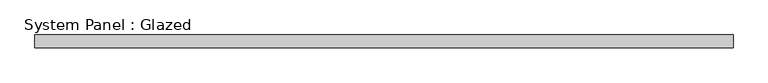
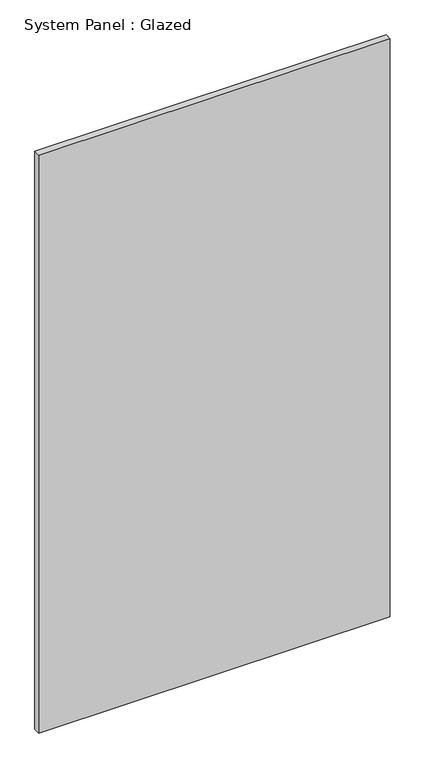
"""IFC4 building model written with IfcOpenShell, lengths in millimetres: plate geometry, System Panel : Glazed."""

from ifc_helpers import new_model, si_unit, origin, origin_with_axes, place, context, project, spatial, polyline, outline, extrude, source, transform, mapped, element, save


def system_panel_glazed_aadce453(model_context):
    return source(origin(), model_context, "Body", "SweptSolid", [
        extrude(outline(polyline([(683.6833332, 19.05), (-683.6833332, 19.05), (-683.6833332, 44.45), (683.6833332, 44.45), (683.6833332, 19.05)])), origin_with_axes(), (0.0, 0.0, 1.0), 2374.9),
    ])


if __name__ == "__main__":
    model = new_model("IFC4")
    model_context = context("Model", 3, world=origin())
    ifc_project = project(units=[si_unit("LENGTHUNIT", "METRE", prefix="MILLI")], contexts=[model_context])
    site = spatial("IfcSite", under=ifc_project)
    building = spatial("IfcBuilding", under=site)
    placement = place(None, origin())
    system_panel_glazed_shape = system_panel_glazed_aadce453(model_context)
    element("IfcPlate", 1, ObjectType="System Panel : Glazed", at=placement, inside=building, context=model_context, shape_type="MappedRepresentation", body=[
        mapped(system_panel_glazed_shape, transform((0.0, 0.0, 0.0), x_axis=(1.0, 0.0, 0.0), y_axis=(0.0, 1.0, 0.0), z_axis=(0.0, 0.0, 1.0))),
    ])
    save(model, "model.ifc")

# Revit data of these elements
# Type "System Panel : Glazed"
#   Construction Type Id = "GSP4R"
#   Analytic Construction = "1/8 in Pilkington single glazing"
#   Visual Light Transmittance = 0.9
#   Solar Heat Gain Coefficient = 0.86
#   Heat Transfer Coefficient (U) = 1.18115 BTU/(h·ft²·°F)
#   Define Thermal Properties by = 1
# Element 1 (IfcPlate, "System Panel : Glazed")
#   Materials on its faces: "Glass"
# Materials
#   "Glass": class "Glass", colour RGB 0 128 192, transparency 0.75, Description = "Soda Lime Glass", Cost = 0
